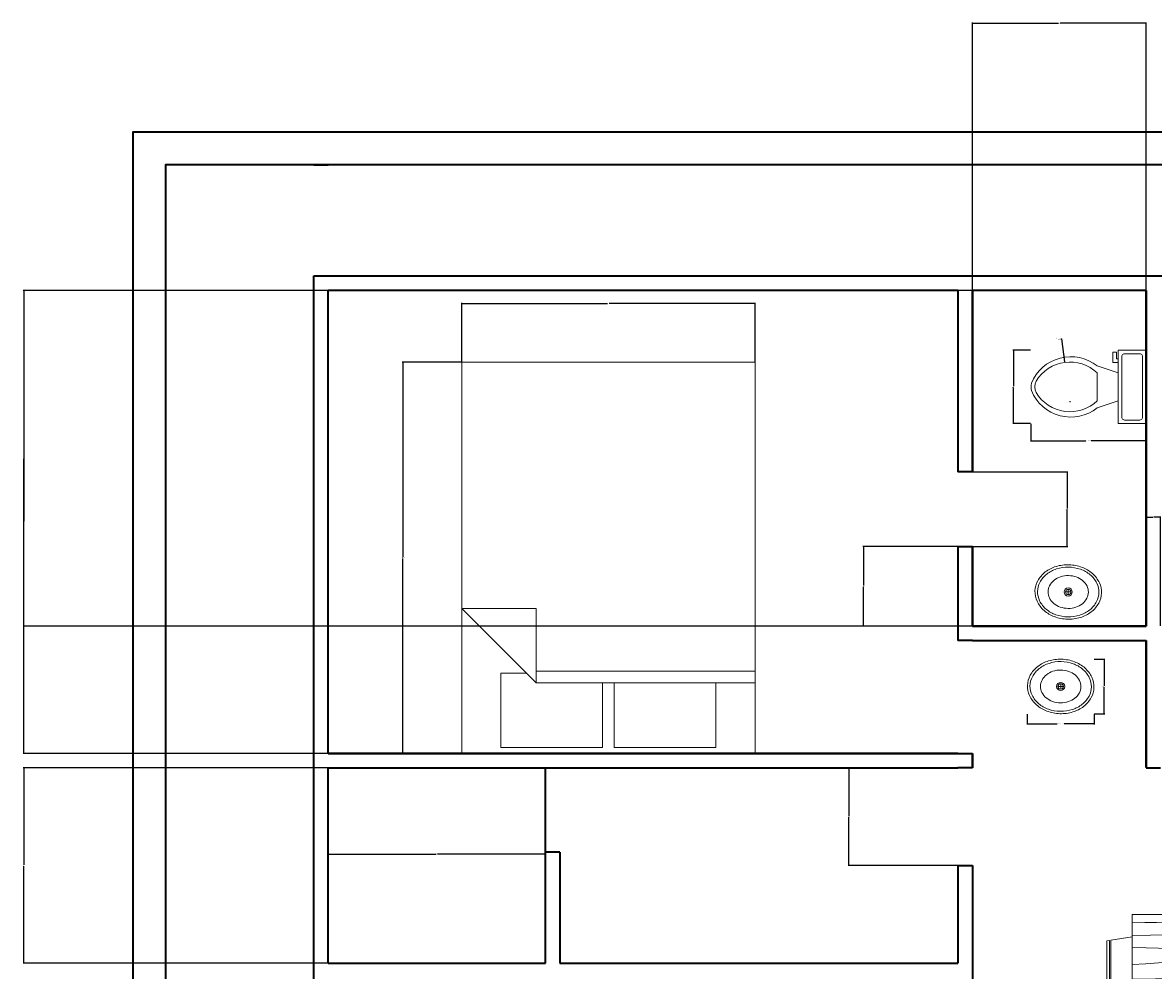
# Model space of a CAD drawing. Units: feet. Extents: x 2335 to 2876, y 491 to 1152.
# Tile 3 of 4: x 2335 to 2648, y 890 to 1152. Entities that reach past the tile are written whole.
import ezdxf

# ---------------------------------------------------------------- set-up
doc = ezdxf.new("R2010")
doc.units = ezdxf.units.FT
for name, color, linetype, lineweight in [('A-ANNO-DIMS', 2, 'Continuous', 18), ('A-FLOR-FIXT', 9, 'Continuous', 18), ('A-FURN', 8, 'Continuous', 18), ('A-WALL', 7, 'Continuous', 35), ('C-PROP', 3, 'Continuous', 35)]:
    doc.layers.add(name, color=color, linetype=linetype, lineweight=lineweight)
doc.styles.get("Standard").update_dxf_attribs({"font": 'arial.ttf'})
doc.dimstyles.get("Standard").update_dxf_attribs({"dimtxt": 0.18, "dimasz": 0.18, "dimexe": 0.18, "dimexo": 0.0625, "dimgap": 0.09, "dimtad": 0, "dimtih": 1, "dimtoh": 1, "dimdec": 4, "dimzin": 0, "dimdsep": 46, "dimlunit": 4, "dimtxsty": 'Standard', "dimcen": 0.09, "dimadec": 0, "dimazin": 0, "dimtfac": 1, "dimtdec": 4, "dimtofl": 0, "dimtmove": 0, "dimatfit": 3, "dimfxl": 1, "dimtolj": 1, "dimtzin": 0, "dimarcsym": 0})

# ---------------------------------------------------------------- blocks, each defined once
blk = doc.blocks.new('Bed - Queen')
for p, q in [((0, -80.00003), (0, 0)), ((0, 0), (59.99999, 0)), ((59.99999, 0), (59.99999, -80.00003)), ((7.99999, -1.2), (28.79998, -1.2)), ((7.99999, -14.4), (7.99999, -1.2)), ((28.79998, -1.2), (28.79998, -14.4)), ((31.19999, -1.2), (51.99999, -1.2)), ((31.19999, -14.4), (31.19999, -1.2)), ((51.99999, -1.2), (51.99999, -16.4)), ((0, -14.4), (44.8, -14.4)), ((59.99999, -29.6), (44.8, -14.4)), ((44.8, -14.4), (44.8, -29.6)), ((44.8, -16.8), (0, -16.8)), ((51.99999, -16.4), (46.79936, -16.4)), ((44.8, -29.6), (59.99999, -29.6)), ((59.99999, -80.00003), (0, -80.00003))]:
    blk.add_line(p, q)
blk = doc.blocks.new('Toilet - top')
for p, q in [((9.5, -6), (9.5, -2)), ((-10, -8.5), (-8, -8.5)), ((-10, -9.5), (-10, -8.5)), ((-7, -9.5), (-10, -9.5)), ((-8, -8.5), (-8, -8)), ((-7, -8), (-7, -9.5)), ((-4, -8), (-6, -14)), ((4, -8), (6, -14)), ((4, -14), (-4, -14))]:
    blk.add_line(p, q)
blk.add_lwpolyline([(10.5, -8), (10.5, 0), (-10.5, 0), (-10.5, -8)], close=True)
for points in [[(-9.5, -2), (-9.5, -6)], [(8.5, -1), (-8.5, -1)], [(-8.5, -7), (8.5, -7)]]:
    blk.add_lwpolyline(points)
for centre, radius, start, end in [((-8.62, -1.88), 0.884, 81.8699, 188.1301), ((8.62, -1.88), 0.884, 351.8699, 98.1301), ((-8.62, -6.12), 0.884, 171.8699, 278.1301), ((8.62, -6.12), 0.884, 261.8699, 8.1301), ((3.52, -21.58), 12.17, 141.4691, 247.9714), ((4.2, -21.82), 11.33, 136.3677, 238.9468), ((-3.52, -21.58), 12.17, 292.0284, 38.5307), ((-4.2, -21.82), 11.33, 301.053, 43.6321), ((0, -27.88), 4, 245.7318, 294.2682), ((0, -29), 4, 254.8605, 285.1395)]:
    blk.add_arc(centre, radius, start, end)
blk = doc.blocks.new('Sink - Oval top')
for p, q in [((-1, 0), (1, 0)), ((0, 1), (0, -1))]:
    blk.add_line(p, q)
for points in [[(-12.23, 0.39, 0.117634), (-11.46, -3.36, 0.104469), (-8.88, -6.8, 0.090016), (-5.08, -9.07, 0.08192), (-0.32, -10.02, 0.08192), (4.49, -9.38, 0.090016), (8.42, -7.36, 0.104469), (11.22, -4.09, 0.117634), (12.23, -0.39, 0.117634), (11.46, 3.36, 0.104469), (8.88, 6.8, 0.090016), (5.08, 9.07, 0.08192), (0.32, 10.02, 0.08192), (-4.49, 9.38, 0.090016), (-8.42, 7.36, 0.104469), (-11.22, 4.09, 0.117634)], [(-11.29, 0.16, 0.118622), (-10.52, -3.25, 0.104678), (-8.07, -6.36, 0.089562), (-4.54, -8.37, 0.081185), (-0.13, -9.15, 0.081185), (4.3, -8.49, 0.089562), (7.89, -6.58, 0.104678), (10.42, -3.55, 0.118622), (11.29, -0.16, 0.118622), (10.52, 3.25, 0.104678), (8.07, 6.36, 0.089562), (4.54, 8.37, 0.081185), (0.13, 9.15, 0.081185), (-4.3, 8.49, 0.089562), (-7.89, 6.58, 0.104678), (-10.42, 3.55, 0.118622)], [(-7.42, 0.08, 0.118283), (-6.91, -2.17, 0.104607), (-5.29, -4.21, 0.089718), (-2.97, -5.53, 0.081436), (-0.07, -6.04, 0.081436), (2.84, -5.59, 0.089718), (5.2, -4.33, 0.104607), (6.86, -2.32, 0.118283), (7.42, -0.08, 0.118283), (6.91, 2.17, 0.104607), (5.29, 4.21, 0.089718), (2.97, 5.53, 0.081436), (0.07, 6.04, 0.081436), (-2.84, 5.59, 0.089718), (-5.2, 4.33, 0.104607), (-6.86, 2.32, 0.118283)]]:
    blk.add_lwpolyline(points, format="xyb", close=True)
for radius in [1.5, 1]:
    blk.add_circle((0, 0), radius)
blk = doc.blocks.new('Dining Set - 36 x 72 in.')
for p, q in [((-22.2343, 26.00059), (-23.4847, 17.99762)), ((-22.2304, 26), (-5.7608, 26)), ((-22, 27.5), (-22.1562, 26.50042)), ((-5.8416, 26.5), (-22.1534, 26.5)), ((-22, 27.5), (-6, 27.5)), ((-5.8437, 26.49966), (-6, 27.5)), ((-4.5152, 17.99762), (-5.7655, 25.99926)), ((5.7657, 26.00059), (4.5153, 17.99762)), ((5.7696, 26), (22.2392, 26)), ((6, 27.5), (5.8438, 26.50042)), ((22.1584, 26.5), (5.8466, 26.5)), ((6, 27.5), (22, 27.5)), ((22.1563, 26.49966), (22, 27.5)), ((23.4848, 17.99762), (22.2345, 25.99926)), ((36, 18), (-36, 18)), ((-36, 18), (-36, -18)), ((36, -18), (36, 18)), ((-44.0006, 8.23428), (-35.9976, 9.48474)), ((44.0006, 8.23428), (35.9976, 9.48474)), ((-45.5, 8), (-44.5004, 8.15617)), ((-45.5, 8), (-45.5, -8)), ((-44.5, -8.15843), (-44.5, 8.15338)), ((-44, 8.23041), (-44, -8.23915)), ((44, 8.23041), (44, -8.23915)), ((44.5, -8.15843), (44.5, 8.15338)), ((45.5, 8), (44.5005, 8.15617)), ((45.5, 8), (45.5, -8)), ((-44.4997, -8.15631), (-45.5, -8)), ((-35.9976, -9.48476), (-43.9993, -8.2345)), ((35.9976, -9.48476), (43.9993, -8.2345)), ((44.4997, -8.15631), (45.5, -8)), ((-36, -18), (36, -18)), ((-22.2343, -26.0006), (-23.4847, -17.99762)), ((-4.5152, -17.99762), (-5.7655, -25.99928)), ((5.7657, -26.0006), (4.5153, -17.99762)), ((23.4848, -17.99762), (22.2345, -25.99928)), ((-22.2304, -26), (-5.7608, -26)), ((-22, -27.5), (-22.1562, -26.50044)), ((-5.8416, -26.5), (-22.1534, -26.5)), ((-22, -27.5), (-6, -27.5)), ((-5.8437, -26.49967), (-6, -27.5)), ((5.7696, -26), (22.2392, -26)), ((6, -27.5), (5.8438, -26.50044)), ((22.1584, -26.5), (5.8466, -26.5)), ((6, -27.5), (22, -27.5)), ((22.1563, -26.49967), (22, -27.5))]:
    blk.add_line(p, q)
for points in [[(-36, 15), (-31.1772, 14.97754), (-26.8079, 14.91406), (-22.8538, 14.81543), (-19.276, 14.6875), (-16.0362, 14.53613), (-13.0957, 14.36718), (-10.4159, 14.18652), (-7.9583, 14), (-5.6904, 13.81315), (-3.6035, 13.63021), (-1.6954, 13.45508), (0.0365, 13.29166), (1.5945, 13.14388), (2.9811, 13.01562), (4.1988, 12.9108), (5.25, 12.83333), (6.1393, 12.78613), (6.8802, 12.76823), (7.4883, 12.77767), (7.9792, 12.8125), (8.3685, 12.87077), (8.6719, 12.95052), (8.9049, 13.0498), (9.0833, 13.16666), (9.2205, 13.29899), (9.3216, 13.44401), (9.3895, 13.59879), (9.4271, 13.76041), (9.4373, 13.92594), (9.4232, 14.09245), (9.3875, 14.257), (9.3333, 14.41666), (9.2638, 14.56917), (9.1836, 14.71484), (9.0975, 14.85465), (9.0104, 14.98958), (8.9272, 15.1206), (8.8529, 15.2487), (8.7922, 15.37483), (8.75, 15.5), (8.7305, 15.62467), (8.7344, 15.74739), (8.7617, 15.86621), (8.8125, 15.97916), (8.8867, 16.08431), (8.9844, 16.17968), (9.1055, 16.26334), (9.25, 16.33333), (9.4189, 16.38802), (9.6172, 16.42708), (9.8506, 16.45052), (10.125, 16.45833), (10.4463, 16.45052), (10.8203, 16.42708), (11.2529, 16.38802), (11.75, 16.33333), (12.3184, 16.26318), (12.9694, 16.17838), (13.7151, 16.07991), (14.5677, 15.96875), (15.5395, 15.84586), (16.6426, 15.71224), (17.8893, 15.56884), (19.2917, 15.41666), (20.859, 15.25667), (22.5879, 15.08984), (24.4721, 14.91715), (26.5052, 14.73958), (28.6809, 14.5581), (30.9929, 14.3737), (33.4347, 14.18733), (36, 14)], [(-36, 10), (-28.9766, 10.14274), (-23.1725, 10.20442), (-18.4241, 10.19775), (-14.5677, 10.13541), (-11.4399, 10.03011), (-8.877, 9.89453), (-6.7154, 9.74137), (-4.7917, 9.58333), (-2.9698, 9.43082), (-1.2246, 9.28515), (0.4415, 9.14534), (2.026, 9.01041), (3.5266, 8.87939), (4.9408, 8.7513), (6.266, 8.62516), (7.5, 8.5), (8.6411, 8.37549), (9.6914, 8.2539), (10.6538, 8.13818), (11.5312, 8.03125), (12.3267, 7.93603), (13.043, 7.85547), (13.6831, 7.79248), (14.25, 7.75), (14.7471, 7.7303), (15.1797, 7.73307), (15.5537, 7.75732), (15.875, 7.80208), (16.1494, 7.86637), (16.3828, 7.94922), (16.5811, 8.04964), (16.75, 8.16666), (16.8944, 8.29915), (17.0143, 8.44531), (17.1089, 8.60319), (17.1771, 8.77083), (17.218, 8.94629), (17.2305, 9.1276), (17.2137, 9.31282), (17.1667, 9.5), (17.0895, 9.6875), (16.987, 9.875), (16.8649, 10.0625), (16.7292, 10.25), (16.5856, 10.4375), (16.4401, 10.625), (16.2985, 10.8125), (16.1667, 11), (16.05, 11.18733), (15.9518, 11.3737), (15.8752, 11.5581), (15.8229, 11.73958), (15.798, 11.91715), (15.8034, 12.08984), (15.842, 12.25667), (15.9167, 12.41666), (16.0295, 12.56836), (16.1784, 12.70833), (16.3605, 12.83268), (16.5729, 12.9375), (16.8127, 13.01888), (17.0768, 13.07291), (17.3625, 13.0957), (17.6667, 13.08333), (17.9894, 13.03312), (18.3418, 12.94726), (18.7382, 12.82918), (19.1927, 12.68229), (19.7195, 12.51001), (20.3327, 12.31575), (21.0465, 12.10294), (21.875, 11.875), (22.8357, 11.63354), (23.959, 11.37304), (25.2786, 11.08618), (26.8282, 10.76562), (28.6414, 10.40405), (30.752, 9.99414), (33.1936, 9.52856), (36, 9)], [(-36, 5.5), (-30.7157, 5.3348), (-26.069, 5.20963), (-21.9946, 5.11767), (-18.4271, 5.05208), (-15.3009, 5.00602), (-12.5508, 4.97265), (-10.1112, 4.94515), (-7.9167, 4.91666), (-5.909, 4.88167), (-4.0586, 4.83984), (-2.3429, 4.79215), (-0.7396, 4.73958), (0.7739, 4.6831), (2.22, 4.6237), (3.6213, 4.56233), (5, 4.5), (6.373, 4.43782), (7.7344, 4.3776), (9.0723, 4.32129), (10.375, 4.27083), (11.6309, 4.22819), (12.8281, 4.19531), (13.9551, 4.17415), (15, 4.16666), (15.954, 4.17448), (16.819, 4.19791), (17.6001, 4.23698), (18.3021, 4.29166), (18.9299, 4.36198), (19.4883, 4.44791), (19.9823, 4.54948), (20.4167, 4.66666), (20.7969, 4.79899), (21.1302, 4.94401), (21.4245, 5.09879), (21.6875, 5.26041), (21.9271, 5.42594), (22.1511, 5.59245), (22.3672, 5.757), (22.5834, 5.91666), (22.8065, 6.06868), (23.0404, 6.21093), (23.2879, 6.34147), (23.5521, 6.45833), (23.8358, 6.55957), (24.142, 6.64323), (24.4735, 6.70735), (24.8334, 6.75), (25.2235, 6.76969), (25.642, 6.76692), (26.0858, 6.74267), (26.5521, 6.69791), (27.0379, 6.63362), (27.5404, 6.55078), (28.0565, 6.45036), (28.5834, 6.33333), (29.1242, 6.19987), (29.7071, 6.04687), (30.3661, 5.87044), (31.1354, 5.66666), (32.0493, 5.43164), (33.142, 5.16146), (34.4475, 4.85221), (36, 4.5)], [(-36, -1), (-30.7915, -0.6591), (-26.0195, -0.38216), (-21.6519, -0.16284), (-17.6563, 0.00521), (-14.0005, 0.12833), (-10.6523, 0.21289), (-7.5796, 0.26522), (-4.75, 0.29166), (-2.134, 0.29793), (0.2878, 0.28711), (2.5317, 0.26163), (4.6146, 0.22396), (6.5529, 0.17651), (8.3633, 0.12174), (10.0623, 0.06209), (11.6667, 0), (13.1899, -0.06201), (14.6341, -0.1211), (15.9982, -0.17432), (17.2813, -0.21875), (18.4823, -0.25147), (19.6003, -0.26953), (20.6343, -0.27002), (21.5834, -0.25), (22.4481, -0.20768), (23.2357, -0.14584), (23.9549, -0.06836), (24.6146, 0.02083), (25.2235, 0.11784), (25.7904, 0.21875), (26.3241, 0.31966), (26.8334, 0.41666), (27.3265, 0.50618), (27.8099, 0.58593), (28.2894, 0.65397), (28.7709, 0.70833), (29.2601, 0.74707), (29.763, 0.76823), (30.2855, 0.76985), (30.8334, 0.75), (31.4088, 0.70784), (31.9994, 0.64713), (32.589, 0.57275), (33.1615, 0.48958), (33.7008, 0.4025), (34.1908, 0.3164), (34.6153, 0.23616), (34.9584, 0.16666), (35.2099, 0.11165), (35.3848, 0.07031), (35.504, 0.04069), (35.5886, 0.02083), (35.6594, 0.00879), (35.7377, 0.0026), (35.8442, 0.00032), (36, 0)], [(-36, -6.5), (-27.1843, -6.31267), (-20.084, -6.1263), (-14.469, -5.9419), (-10.1094, -5.76042), (-6.7752, -5.58285), (-4.2363, -5.41016), (-2.2629, -5.24333), (-0.625, -5.08334), (0.8708, -4.93099), (2.2715, -4.78646), (3.5872, -4.64974), (4.8281, -4.52084), (6.0046, -4.39974), (7.127, -4.28646), (8.2053, -4.18099), (9.25, -4.08334), (10.2705, -3.99382), (11.2734, -3.91407), (12.2647, -3.84603), (13.25, -3.79167), (14.2354, -3.75293), (15.2266, -3.73177), (16.2295, -3.73015), (17.25, -3.75), (18.2912, -3.79248), (19.3451, -3.85547), (20.4009, -3.93604), (21.4479, -4.03125), (22.4754, -4.13819), (23.4727, -4.25391), (24.4289, -4.37549), (25.3334, -4.5), (26.1785, -4.62492), (26.9694, -4.74935), (27.7145, -4.87281), (28.4219, -4.99479), (29.1, -5.11483), (29.7572, -5.23242), (30.4016, -5.34709), (31.0417, -5.45834), (31.6837, -5.56437), (32.3262, -5.65821), (32.9658, -5.73153), (33.599, -5.77604), (34.2224, -5.78345), (34.8327, -5.74545), (35.4264, -5.65373), (36, -5.5)], [(-36, -10), (-26.4022, -9.81299), (-18.4675, -9.62891), (-11.9839, -9.45069), (-6.7396, -9.28125), (-2.5226, -9.12354), (0.8789, -8.98047), (3.6769, -8.85498), (6.0833, -8.75), (8.2767, -8.66765), (10.3021, -8.60677), (12.1712, -8.56543), (13.8958, -8.54167), (15.4876, -8.53353), (16.9583, -8.53907), (18.3197, -8.55632), (19.5834, -8.58334), (20.7616, -8.61841), (21.8685, -8.66081), (22.9188, -8.71004), (23.9271, -8.76563), (24.9081, -8.82707), (25.8763, -8.89388), (26.8465, -8.96558), (27.8334, -9.04167), (28.8474, -9.12118), (29.8828, -9.20117), (30.93, -9.27824), (31.9792, -9.34896), (33.0205, -9.40991), (34.0443, -9.45768), (35.0407, -9.48885), (36, -9.5)], [(-36, -14.5), (-30.0881, -14.33513), (-25.0332, -14.21224), (-20.7312, -14.12647), (-17.0781, -14.07292), (-13.97, -14.04671), (-11.3027, -14.04297), (-8.9724, -14.05681), (-6.875, -14.08334), (-4.9224, -14.11833), (-3.0905, -14.16016), (-1.3709, -14.20785), (0.2448, -14.26042), (1.7647, -14.3169), (3.1973, -14.3763), (4.5507, -14.43767), (5.8333, -14.5), (7.0554, -14.5621), (8.235, -14.62175), (9.3922, -14.67652), (10.5469, -14.72396), (11.7192, -14.76164), (12.929, -14.78711), (14.1965, -14.79794), (15.5417, -14.79167), (16.9933, -14.76424), (18.6152, -14.70508), (20.4804, -14.60197), (22.6615, -14.44271), (25.2312, -14.21509), (28.2624, -13.9069), (31.8277, -13.50594), (36, -13)]]:
    blk.add_lwpolyline(points)
blk = doc.blocks.new('*D8')
at = {"layer": 'A-ANNO-DIMS', "color": 0, "lineweight": -2, "transparency": 16777216}
for p, q in [((2456.6, 1057.92), (2440.26, 1057.92)), ((2440.44, 1057.74), (2440.44, 1004.04)), ((2440.44, 949.98), (2440.44, 1003.68)), ((2456.6, 949.8), (2440.26, 949.8))]:
    blk.add_line(p, q, dxfattribs=at)
at = {"layer": 'A-ANNO-DIMS', "color": 0, "transparency": 16777216}
for points in [[(2440.41, 1057.74), (2440.47, 1057.74), (2440.44, 1057.92)], [(2440.41, 949.98), (2440.47, 949.98), (2440.44, 949.8)]]:
    blk.add_solid(points, dxfattribs=at)
at = {"layer": 'Defpoints', "color": 0, "transparency": 16777216}
for p in [(2456.66, 1057.92), (2440.44, 949.8), (2456.66, 949.8)]:
    blk.add_point(p, dxfattribs=at)
at = {"layer": 'A-ANNO-DIMS', "color": 0, "transparency": 16777216, "insert": (2440.44, 1003.86), "char_height": 0.18, "attachment_point": 5}
blk.add_mtext('\\A1;BED 108', dxfattribs=at)
blk = doc.blocks.new('*D9')
at = {"layer": 'A-ANNO-DIMS', "color": 0, "lineweight": -2, "transparency": 16777216}
for p, q in [((2456.66, 1057.98), (2456.66, 1074.31)), ((2456.84, 1074.13), (2497, 1074.13)), ((2537.57, 1074.13), (2497.41, 1074.13)), ((2537.75, 1057.98), (2537.75, 1074.31))]:
    blk.add_line(p, q, dxfattribs=at)
at = {"layer": 'A-ANNO-DIMS', "color": 0, "transparency": 16777216}
for points in [[(2456.84, 1074.16), (2456.84, 1074.1), (2456.66, 1074.13)], [(2537.57, 1074.16), (2537.57, 1074.1), (2537.75, 1074.13)]]:
    blk.add_solid(points, dxfattribs=at)
at = {"layer": 'Defpoints', "color": 0, "transparency": 16777216}
for p in [(2456.66, 1074.13), (2456.66, 1057.92), (2537.75, 1057.92)]:
    blk.add_point(p, dxfattribs=at)
at = {"layer": 'A-ANNO-DIMS', "color": 0, "transparency": 16777216, "insert": (2497.21, 1074.13), "char_height": 0.18, "attachment_point": 5}
blk.add_mtext('\\A1;81', dxfattribs=at)
blk = doc.blocks.new('*D12')
at = {"layer": 'A-ANNO-DIMS', "color": 0, "lineweight": -2, "transparency": 16777216}
for p, q in [((2612.96, 960.67), (2612.96, 957.78)), ((2631.41, 960.67), (2631.41, 957.78)), ((2613.14, 957.96), (2621.25, 957.96)), ((2631.23, 957.96), (2623.12, 957.96))]:
    blk.add_line(p, q, dxfattribs=at)
at = {"layer": 'A-ANNO-DIMS', "color": 0, "transparency": 16777216}
for points in [[(2613.14, 957.99), (2613.14, 957.93), (2612.96, 957.96)], [(2631.23, 957.99), (2631.23, 957.93), (2631.41, 957.96)]]:
    blk.add_solid(points, dxfattribs=at)
at = {"layer": 'Defpoints', "color": 0, "transparency": 16777216}
for p in [(2612.96, 960.73), (2631.41, 960.73), (2631.41, 957.96)]:
    blk.add_point(p, dxfattribs=at)
at = {"layer": 'A-ANNO-DIMS', "color": 0, "transparency": 16777216, "insert": (2622.19, 957.96), "char_height": 0.18, "attachment_point": 5}
blk.add_mtext('\\A1;BASIN 18 TYP.', dxfattribs=at)
blk = doc.blocks.new('*D13')
at = {"layer": 'A-ANNO-DIMS', "color": 0, "lineweight": -2, "transparency": 16777216}
for p, q in [((2631.47, 975.86), (2634.36, 975.86)), ((2634.18, 975.68), (2634.18, 968.48)), ((2634.18, 960.91), (2634.18, 968.12)), ((2631.47, 960.73), (2634.36, 960.73))]:
    blk.add_line(p, q, dxfattribs=at)
at = {"layer": 'A-ANNO-DIMS', "color": 0, "transparency": 16777216}
for points in [[(2634.15, 975.68), (2634.21, 975.68), (2634.18, 975.86)], [(2634.15, 960.91), (2634.21, 960.91), (2634.18, 960.73)]]:
    blk.add_solid(points, dxfattribs=at)
at = {"layer": 'Defpoints', "color": 0, "transparency": 16777216}
for p in [(2631.41, 975.86), (2634.18, 975.86), (2631.41, 960.73)]:
    blk.add_point(p, dxfattribs=at)
at = {"layer": 'A-ANNO-DIMS', "color": 0, "transparency": 16777216, "insert": (2634.18, 968.3), "char_height": 0.18, "attachment_point": 5}
blk.add_mtext('\\A1;15 TYP.', dxfattribs=at)
blk = doc.blocks.new('*D14')
at = {"layer": 'A-ANNO-DIMS', "color": 0, "lineweight": -2, "transparency": 16777216}
for p, q in [((2613.94, 1040.92), (2613.94, 1036.03)), ((2645.8, 1040.92), (2645.8, 1036.03)), ((2614.12, 1036.21), (2629.09, 1036.21)), ((2645.62, 1036.21), (2630.64, 1036.21))]:
    blk.add_line(p, q, dxfattribs=at)
at = {"layer": 'A-ANNO-DIMS', "color": 0, "transparency": 16777216}
for points in [[(2614.12, 1036.24), (2614.12, 1036.18), (2613.94, 1036.21)], [(2645.62, 1036.24), (2645.62, 1036.18), (2645.8, 1036.21)]]:
    blk.add_solid(points, dxfattribs=at)
at = {"layer": 'Defpoints', "color": 0, "transparency": 16777216}
for p in [(2613.94, 1040.98), (2645.8, 1040.98), (2645.8, 1036.21)]:
    blk.add_point(p, dxfattribs=at)
at = {"layer": 'A-ANNO-DIMS', "color": 0, "transparency": 16777216, "insert": (2629.87, 1036.21), "char_height": 0.18, "attachment_point": 5}
blk.add_mtext('\\A1;WC 32 TYP.', dxfattribs=at)
blk = doc.blocks.new('*D15')
at = {"layer": 'A-ANNO-DIMS', "color": 0, "lineweight": -2, "transparency": 16777216}
for p, q in [((2613.87, 1061.23), (2608.98, 1061.23)), ((2609.16, 1061.05), (2609.16, 1051.29)), ((2609.16, 1041.16), (2609.16, 1050.93)), ((2613.87, 1040.98), (2608.98, 1040.98))]:
    blk.add_line(p, q, dxfattribs=at)
at = {"layer": 'A-ANNO-DIMS', "color": 0, "transparency": 16777216}
for points in [[(2609.13, 1061.05), (2609.19, 1061.05), (2609.16, 1061.23)], [(2609.13, 1041.16), (2609.19, 1041.16), (2609.16, 1040.98)]]:
    blk.add_solid(points, dxfattribs=at)
at = {"layer": 'Defpoints', "color": 0, "transparency": 16777216}
for p in [(2613.94, 1061.23), (2609.16, 1040.98), (2613.94, 1040.98)]:
    blk.add_point(p, dxfattribs=at)
at = {"layer": 'A-ANNO-DIMS', "color": 0, "transparency": 16777216, "insert": (2609.16, 1051.11), "char_height": 0.18, "attachment_point": 5}
blk.add_mtext('\\A1;20 TYP.', dxfattribs=at)
blk = doc.blocks.new('*D50')
at = {"layer": 'A-ANNO-DIMS', "color": 0, "lineweight": -2, "transparency": 16777216}
for p, q in [((2419.73, 945.8), (2335.47, 945.8)), ((2335.65, 945.62), (2335.65, 918.98)), ((2335.65, 891.98), (2335.65, 918.62)), ((2419.73, 891.8), (2335.47, 891.8))]:
    blk.add_line(p, q, dxfattribs=at)
at = {"layer": 'A-ANNO-DIMS', "color": 0, "transparency": 16777216}
for points in [[(2335.62, 945.62), (2335.68, 945.62), (2335.65, 945.8)], [(2335.62, 891.98), (2335.68, 891.98), (2335.65, 891.8)]]:
    blk.add_solid(points, dxfattribs=at)
at = {"layer": 'Defpoints', "color": 0, "transparency": 16777216}
for p in [(2335.65, 945.8), (2419.8, 945.8), (2419.8, 891.8)]:
    blk.add_point(p, dxfattribs=at)
at = {"layer": 'A-ANNO-DIMS', "color": 0, "transparency": 16777216, "insert": (2335.65, 918.8), "char_height": 0.18, "attachment_point": 5}
blk.add_mtext('\\A1;54', dxfattribs=at)
blk = doc.blocks.new('*D51')
at = {"layer": 'A-ANNO-DIMS', "color": 0, "lineweight": -2, "transparency": 16777216}
for p, q in [((2419.8, 891.86), (2419.8, 922.13)), ((2419.98, 921.95), (2449.58, 921.95)), ((2479.62, 921.95), (2450.02, 921.95)), ((2479.8, 891.86), (2479.8, 922.13))]:
    blk.add_line(p, q, dxfattribs=at)
at = {"layer": 'A-ANNO-DIMS', "color": 0, "transparency": 16777216}
for points in [[(2419.98, 921.98), (2419.98, 921.92), (2419.8, 921.95)], [(2479.62, 921.98), (2479.62, 921.92), (2479.8, 921.95)]]:
    blk.add_solid(points, dxfattribs=at)
at = {"layer": 'Defpoints', "color": 0, "transparency": 16777216}
for p in [(2479.8, 921.95), (2419.8, 891.8), (2479.8, 891.8)]:
    blk.add_point(p, dxfattribs=at)
at = {"layer": 'A-ANNO-DIMS', "color": 0, "transparency": 16777216, "insert": (2449.8, 921.95), "char_height": 0.18, "attachment_point": 5}
blk.add_mtext('\\A1;60', dxfattribs=at)
blk = doc.blocks.new('*D52')
at = {"layer": 'A-ANNO-DIMS', "color": 0, "lineweight": -2, "transparency": 16777216}
for p, q in [((2593.73, 945.8), (2563.47, 945.8)), ((2563.65, 945.62), (2563.65, 932.48)), ((2563.65, 918.98), (2563.65, 932.12)), ((2593.73, 918.8), (2563.47, 918.8))]:
    blk.add_line(p, q, dxfattribs=at)
at = {"layer": 'A-ANNO-DIMS', "color": 0, "transparency": 16777216}
for points in [[(2563.62, 945.62), (2563.68, 945.62), (2563.65, 945.8)], [(2563.62, 918.98), (2563.68, 918.98), (2563.65, 918.8)]]:
    blk.add_solid(points, dxfattribs=at)
at = {"layer": 'Defpoints', "color": 0, "transparency": 16777216}
for p in [(2563.65, 945.8), (2593.8, 945.8), (2593.8, 918.8)]:
    blk.add_point(p, dxfattribs=at)
at = {"layer": 'A-ANNO-DIMS', "color": 0, "transparency": 16777216, "insert": (2563.65, 932.3), "char_height": 0.18, "attachment_point": 5}
blk.add_mtext('\\A1;27', dxfattribs=at)
blk = doc.blocks.new('*D53')
at = {"layer": 'A-ANNO-DIMS', "color": 0, "lineweight": -2, "transparency": 16777216}
for p, q in [((2419.74, 1077.8), (2335.47, 1077.8)), ((2335.65, 1077.62), (2335.65, 1013.98)), ((2335.65, 949.98), (2335.65, 1013.62)), ((2419.73, 949.8), (2335.47, 949.8))]:
    blk.add_line(p, q, dxfattribs=at)
at = {"layer": 'A-ANNO-DIMS', "color": 0, "transparency": 16777216}
for points in [[(2335.62, 1077.62), (2335.68, 1077.62), (2335.65, 1077.8)], [(2335.62, 949.98), (2335.68, 949.98), (2335.65, 949.8)]]:
    blk.add_solid(points, dxfattribs=at)
at = {"layer": 'Defpoints', "color": 0, "transparency": 16777216}
for p in [(2335.65, 1077.8), (2419.8, 1077.8), (2419.8, 949.8)]:
    blk.add_point(p, dxfattribs=at)
at = {"layer": 'A-ANNO-DIMS', "color": 0, "transparency": 16777216, "insert": (2335.65, 1013.8), "char_height": 0.18, "attachment_point": 5}
blk.add_mtext('\\A1;128', dxfattribs=at)
blk = doc.blocks.new('*D55')
at = {"layer": 'A-ANNO-DIMS', "color": 0, "lineweight": -2, "transparency": 16777216}
for p, q in [((2597.8, 1077.86), (2597.8, 1151.82)), ((2597.98, 1151.64), (2621.57, 1151.64)), ((2645.62, 1151.64), (2622.02, 1151.64)), ((2645.8, 1077.86), (2645.8, 1151.82))]:
    blk.add_line(p, q, dxfattribs=at)
at = {"layer": 'A-ANNO-DIMS', "color": 0, "transparency": 16777216}
for points in [[(2597.98, 1151.67), (2597.98, 1151.61), (2597.8, 1151.64)], [(2645.62, 1151.67), (2645.62, 1151.61), (2645.8, 1151.64)]]:
    blk.add_solid(points, dxfattribs=at)
at = {"layer": 'Defpoints', "color": 0, "transparency": 16777216}
for p in [(2645.8, 1151.64), (2597.8, 1077.8), (2645.8, 1077.8)]:
    blk.add_point(p, dxfattribs=at)
at = {"layer": 'A-ANNO-DIMS', "color": 0, "transparency": 16777216, "insert": (2621.8, 1151.64), "char_height": 0.18, "attachment_point": 5}
blk.add_mtext('\\A1;48', dxfattribs=at)
blk = doc.blocks.new('*D57')
at = {"layer": 'A-ANNO-DIMS', "color": 0, "lineweight": -2, "transparency": 16777216}
for p, q in [((2645.8, 985.02), (2645.8, 1015.28)), ((2645.98, 1015.1), (2647.65, 1015.1)), ((2649.62, 1015.1), (2647.95, 1015.1)), ((2649.8, 985.02), (2649.8, 1015.28))]:
    blk.add_line(p, q, dxfattribs=at)
at = {"layer": 'A-ANNO-DIMS', "color": 0, "transparency": 16777216}
for points in [[(2645.98, 1015.13), (2645.98, 1015.07), (2645.8, 1015.1)], [(2649.62, 1015.13), (2649.62, 1015.07), (2649.8, 1015.1)]]:
    blk.add_solid(points, dxfattribs=at)
at = {"layer": 'Defpoints', "color": 0, "transparency": 16777216}
for p in [(2649.8, 1015.1), (2645.8, 984.95), (2649.8, 984.95)]:
    blk.add_point(p, dxfattribs=at)
at = {"layer": 'A-ANNO-DIMS', "color": 0, "transparency": 16777216, "insert": (2647.8, 1015.1), "char_height": 0.18, "attachment_point": 5}
blk.add_mtext('\\A1;4', dxfattribs=at)
blk = doc.blocks.new('*D58')
at = {"layer": 'A-ANNO-DIMS', "color": 0, "lineweight": -2, "transparency": 16777216}
for p, q in [((2597.73, 1077.8), (2335.47, 1077.8)), ((2335.65, 1077.62), (2335.65, 1031.56)), ((2335.65, 985.13), (2335.65, 1031.19)), ((2597.73, 984.95), (2335.47, 984.95))]:
    blk.add_line(p, q, dxfattribs=at)
at = {"layer": 'A-ANNO-DIMS', "color": 0, "transparency": 16777216}
for points in [[(2335.62, 1077.62), (2335.68, 1077.62), (2335.65, 1077.8)], [(2335.62, 985.13), (2335.68, 985.13), (2335.65, 984.95)]]:
    blk.add_solid(points, dxfattribs=at)
at = {"layer": 'Defpoints', "color": 0, "transparency": 16777216}
for p in [(2335.65, 1077.8), (2597.8, 1077.8), (2597.8, 984.95)]:
    blk.add_point(p, dxfattribs=at)
at = {"layer": 'A-ANNO-DIMS', "color": 0, "transparency": 16777216, "insert": (2335.65, 1031.38), "char_height": 0.18, "attachment_point": 5}
blk.add_mtext('\\A1;92.84', dxfattribs=at)
blk = doc.blocks.new('*D64')
at = {"layer": 'A-ANNO-DIMS', "color": 0, "lineweight": -2, "transparency": 16777216}
for p, q in [((2593.86, 1027.59), (2624.13, 1027.59)), ((2623.95, 1027.41), (2623.95, 1017.47)), ((2623.95, 1007.17), (2623.95, 1017.11)), ((2593.86, 1006.99), (2624.13, 1006.99))]:
    blk.add_line(p, q, dxfattribs=at)
at = {"layer": 'A-ANNO-DIMS', "color": 0, "transparency": 16777216}
for points in [[(2623.92, 1027.41), (2623.98, 1027.41), (2623.95, 1027.59)], [(2623.92, 1007.17), (2623.98, 1007.17), (2623.95, 1006.99)]]:
    blk.add_solid(points, dxfattribs=at)
at = {"layer": 'Defpoints', "color": 0, "transparency": 16777216}
for p in [(2593.8, 1027.59), (2593.8, 1006.99), (2623.95, 1006.99)]:
    blk.add_point(p, dxfattribs=at)
at = {"layer": 'A-ANNO-DIMS', "color": 0, "transparency": 16777216, "insert": (2623.95, 1017.29), "char_height": 0.18, "attachment_point": 5}
blk.add_mtext('\\A1;20.597', dxfattribs=at)
blk = doc.blocks.new('*D67')
at = {"layer": 'A-ANNO-DIMS', "color": 0, "lineweight": -2, "transparency": 16777216}
for p, q in [((2597.73, 1006.99), (2567.47, 1006.99)), ((2567.65, 1006.81), (2567.65, 996.16)), ((2567.65, 985.13), (2567.65, 995.79)), ((2597.73, 984.95), (2567.47, 984.95))]:
    blk.add_line(p, q, dxfattribs=at)
at = {"layer": 'A-ANNO-DIMS', "color": 0, "transparency": 16777216}
for points in [[(2567.62, 1006.81), (2567.68, 1006.81), (2567.65, 1006.99)], [(2567.62, 985.13), (2567.68, 985.13), (2567.65, 984.95)]]:
    blk.add_solid(points, dxfattribs=at)
at = {"layer": 'Defpoints', "color": 0, "transparency": 16777216}
for p in [(2567.65, 1006.99), (2597.8, 1006.99), (2597.8, 984.95)]:
    blk.add_point(p, dxfattribs=at)
at = {"layer": 'A-ANNO-DIMS', "color": 0, "transparency": 16777216, "insert": (2567.65, 995.97), "char_height": 0.18, "attachment_point": 5}
blk.add_mtext('\\A1;22.04', dxfattribs=at)
blk = doc.blocks.new('*D69')
at = {"layer": 'A-ANNO-DIMS', "color": 0, "lineweight": -2, "transparency": 16777216}
for p, q in [((2622.25, 1064.38), (2622.43, 1064.38)), ((2622.43, 1064.38), (2623.28, 1058.06)), ((2624.67, 1047.06), (2624.85, 1047.06)), ((2624.76, 1046.97), (2624.76, 1047.15))]:
    blk.add_line(p, q, dxfattribs=at)
at = {"layer": 'A-ANNO-DIMS', "color": 0, "transparency": 16777216}
blk.add_solid([(2623.31, 1058.07), (2623.25, 1058.06), (2623.31, 1057.88)], dxfattribs=at)
at = {"layer": 'Defpoints', "color": 0, "transparency": 16777216}
for p in [(2623.31, 1057.88), (2624.76, 1047.06)]:
    blk.add_point(p, dxfattribs=at)
at = {"layer": 'A-ANNO-DIMS', "color": 0, "transparency": 16777216, "insert": (2621.51, 1064.38), "char_height": 0.18, "attachment_point": 5}
blk.add_mtext('\\A1;4X R10.923', dxfattribs=at)

msp = doc.modelspace()

# ---------------------------------------------------------------- linework, layer by layer
at = {"layer": 'A-WALL'}
for p, q in [((2415.7974, 855.7568), (2415.7974, 1081.7975)), ((2415.7974, 1081.7975), (2697.7974, 1081.7975)), ((2593.7974, 1077.7977), (2419.7973, 1077.798)), ((2419.7974, 949.7975), (2419.7976, 1077.798)), ((2593.7974, 1077.7977), (2593.7974, 1027.5899)), ((2593.7974, 1077.7977), (2593.7974, 1027.5899)), ((2593.7974, 1077.7977), (2593.7974, 1027.5899)), ((2597.7974, 1077.7977), (2597.7974, 1027.5899)), ((2645.7974, 1077.7976), (2597.7974, 1077.7977)), ((2597.7974, 1027.5899), (2597.7974, 1077.7977)), ((2645.7974, 984.9529), (2645.7974, 1077.7976)), ((2645.7974, 1077.7976), (2645.7974, 984.9529)), ((2645.7974, 1077.7976), (2645.7974, 984.9529)), ((2645.7974, 1077.7976), (2645.7974, 984.9529)), ((2597.7974, 1027.5899), (2593.7974, 1027.5899)), ((2593.7974, 1006.9934), (2597.7974, 1006.9934)), ((2593.7974, 1006.9934), (2593.7974, 980.9529)), ((2593.7974, 1006.9934), (2593.7974, 980.9529)), ((2593.7974, 1006.9934), (2593.7974, 980.9529)), ((2597.7974, 984.9529), (2597.7974, 1006.9934)), ((2597.7974, 1006.9934), (2597.7974, 984.9529)), ((2645.7974, 984.9529), (2597.7974, 984.9529)), ((2597.7974, 984.9529), (2645.7974, 984.9529)), ((2645.7974, 984.9529), (2597.7974, 984.9529)), ((2597.7974, 984.9529), (2645.7974, 984.9529)), ((2597.7974, 980.9529), (2593.7974, 980.9529)), ((2597.7974, 980.9529), (2645.7974, 980.9529)), ((2597.7974, 980.9529), (2645.7974, 980.9529)), ((2597.7974, 980.9529), (2645.7974, 980.9529)), ((2645.7974, 945.9689), (2645.7974, 980.9529)), ((2645.7974, 980.9529), (2645.7974, 949.7975)), ((2645.7974, 980.9529), (2645.7974, 945.7975)), ((2645.7974, 980.9529), (2645.7974, 949.7975)), ((2593.7974, 949.7975), (2419.7974, 949.7975)), ((2419.7974, 949.7975), (2593.7974, 949.7975)), ((2593.7974, 949.7975), (2419.7974, 949.7975)), ((2593.7974, 949.7975), (2597.7974, 949.7975)), ((2597.7974, 945.7975), (2597.7974, 949.7975)), ((2597.7974, 949.7975), (2597.7974, 945.7975)), ((2597.7974, 949.7975), (2597.7974, 945.7975)), ((2419.7969, 891.7975), (2419.7969, 945.7975)), ((2419.7974, 945.7975), (2593.7974, 945.7975)), ((2419.7974, 945.7975), (2593.7974, 945.7975)), ((2479.7974, 891.7975), (2479.7974, 945.7975)), ((2597.7974, 945.7975), (2593.7974, 945.7975)), ((2645.7974, 945.7975), (2649.7974, 945.7975)), ((2483.7974, 922.4546), (2479.7974, 922.4546)), ((2483.7974, 922.4546), (2483.7974, 891.7975)), ((2593.7974, 918.7975), (2593.7974, 891.7975)), ((2593.7974, 918.7975), (2597.7974, 918.7975)), ((2597.7974, 918.7975), (2597.7974, 614.2261)), ((2419.7974, 891.7975), (2479.7974, 891.7975)), ((2483.7974, 891.7975), (2593.7974, 891.7975))]:
    msp.add_line(p, q, dxfattribs=at)
at = {"layer": 'C-PROP'}
for p, q in [((2374.7967, 1112.4872), (2374.7967, 1081.7975)), ((2415.7974, 1112.4872), (2419.7974, 1112.4872))]:
    msp.add_line(p, q, dxfattribs=at)
msp.add_lwpolyline([(2845.7967, 521.4872), (2845.7967, 1121.4872), (2365.7967, 1121.4872), (2365.7967, 521.4872)], close=True, dxfattribs=at)
msp.add_lwpolyline([(2697.7974, 1112.4872), (2374.7967, 1112.4872), (2374.7967, 530.4872), (2593.7974, 530.4872)], dxfattribs=at)

# ---------------------------------------------------------------- block references
at = {"layer": 'A-FLOR-FIXT', "xscale": 0.9641315578102057, "yscale": 0.9641315578102057, "zscale": 0.9641315578102057, "rotation": 270}
msp.add_blockref('Toilet - top', (2645.7974, 1051.1075), dxfattribs=at)
at = {"layer": 'A-FLOR-FIXT', "xscale": 0.7514563269629554, "yscale": 0.7514563269629554, "zscale": 0.7514563269629554}
for p in [(2624.2621, 994.4081), (2622.1863, 968.2974)]:
    msp.add_blockref('Sink - Oval top', p, dxfattribs=at)
at = {"layer": 'A-FURN', "xscale": 1.35149041109511, "yscale": 1.35149041109511, "zscale": 1.35149041109511, "rotation": 180}
msp.add_blockref('Bed - Queen', (2537.7499, 949.7975), dxfattribs=at)
at = {"layer": 'A-FURN', "xscale": 0.7311477324397611, "yscale": 0.7311477324397611, "zscale": 0.7311477324397611}
msp.add_blockref('Dining Set - 36 x 72 in.', (2668.2264, 892.1257), dxfattribs=at)

# ---------------------------------------------------------------- dimensions: what is measured, and where the dimension line sits
at = {"layer": 'A-ANNO-DIMS'}
for base, p1, p2, picture, middle in [((2645.7974, 1151.6372), (2597.7974, 1077.7977), (2645.7974, 1077.7976), '*D55', (2621.7974, 1151.6372)), ((2649.7974, 1015.1029), (2645.7974, 984.9529), (2649.7974, 984.9529), '*D57', (2647.7974, 1015.1029)), ((2479.7974, 921.9475), (2419.7974, 891.7975), (2479.7974, 891.7975), '*D51', (2449.7974, 921.9475))]:
    dim = msp.add_linear_dim(base=base, p1=p1, p2=p2, dimstyle='Standard', override={"dimdec": 0, "dimlfac": 1, "dimrnd": 0, "dimzin": 0, "dimdsep": 46, "dimlunit": 2}, dxfattribs=at)
    dim.commit()
    dim.dimension.update_dxf_attribs({"geometry": picture, "text_midpoint": middle})
for base, p1, p2, angle, override, picture, middle in [((2335.6467, 1077.7977), (2597.7974, 984.9529), (2597.7974, 1077.7977), 90, {"dimdec": 2, "dimlfac": 1, "dimrnd": 0, "dimzin": 0, "dimdsep": 46, "dimlunit": 2}, '*D58', (2335.6467, 1031.3753)), ((2335.6467, 1077.798), (2419.7974, 949.7975), (2419.7976, 1077.798), 90, {"dimdec": 0, "dimlfac": 1, "dimrnd": 0, "dimzin": 0, "dimdsep": 46, "dimlunit": 2}, '*D53', (2335.6467, 1013.7978)), ((2456.6605, 1074.1347), (2537.7499, 1057.9168), (2456.6605, 1057.9168), 180, {"dimdec": 0, "dimlfac": 1, "dimrnd": 0, "dimzin": 0, "dimdsep": 46, "dimlunit": 2}, '*D9', (2497.2052, 1074.1347)), ((2623.94739, 1006.99339), (2593.79739, 1027.58992), (2593.79739, 1006.99339), 270, {"dimdec": 3, "dimlfac": 1, "dimrnd": 0, "dimzin": 0, "dimdsep": 46, "dimlunit": 2}, '*D64', (2623.94739, 1017.29165)), ((2567.6474, 1006.9934), (2597.7974, 984.9529), (2597.7974, 1006.9934), 90, {"dimdec": 2, "dimlfac": 1, "dimrnd": 0, "dimzin": 0, "dimdsep": 46, "dimlunit": 2}, '*D67', (2567.6474, 995.9731)), ((2335.6467, 945.7975), (2419.7974, 891.7975), (2419.7974, 945.7975), 90, {"dimdec": 0, "dimlfac": 1, "dimrnd": 0, "dimzin": 0, "dimdsep": 46, "dimlunit": 2}, '*D50', (2335.6467, 918.7975)), ((2563.6474, 945.7975), (2593.7974, 918.7975), (2593.7974, 945.7975), 90, {"dimdec": 0, "dimlfac": 1, "dimrnd": 0, "dimzin": 0, "dimdsep": 46, "dimlunit": 2}, '*D52', (2563.6474, 932.2975))]:
    dim = msp.add_linear_dim(base=base, p1=p1, p2=p2, angle=angle, dimstyle='Standard', override=override, dxfattribs=at)
    dim.commit()
    dim.dimension.update_dxf_attribs({"geometry": picture, "text_midpoint": middle})
dim = msp.add_radius_dim(center=(2624.7625, 1047.0582), mpoint=(2623.307, 1057.8836), text='4X <>', dimstyle='Standard', override={"dimdec": 3, "dimlfac": 1, "dimrnd": 0, "dimzin": 0, "dimdsep": 46, "dimlunit": 2}, dxfattribs=at)
dim.commit()
dim.dimension.update_dxf_attribs({"geometry": '*D69', "text_midpoint": (2621.507, 1064.3789), "dimtype": 164})
for base, p1, p2, angle, text, picture, middle in [((2609.1573, 1040.9842), (2613.9365, 1061.2309), (2613.9365, 1040.9842), 270, '<> TYP.', '*D15', (2609.1573, 1051.1075)), ((2440.4426, 949.7975), (2456.6605, 1057.9168), (2456.6605, 949.7975), 270, 'BED <>', '*D8', (2440.4426, 1003.8571)), ((2634.1781, 975.8633), (2631.4107, 960.7315), (2631.4107, 975.8633), 90, '<> TYP.', '*D13', (2634.1781, 968.2974))]:
    dim = msp.add_linear_dim(base=base, p1=p1, p2=p2, angle=angle, text=text, dimstyle='Standard', override={"dimdec": 0, "dimlfac": 1, "dimrnd": 0, "dimzin": 0, "dimdsep": 46, "dimlunit": 2}, dxfattribs=at)
    dim.commit()
    dim.dimension.update_dxf_attribs({"geometry": picture, "text_midpoint": middle})
for base, p1, p2, text, picture, middle in [((2645.7974, 1036.205), (2613.9365, 1040.9842), (2645.7974, 1040.9842), 'WC <> TYP.', '*D14', (2629.8669, 1036.205)), ((2631.4107, 957.9642), (2612.9618, 960.7315), (2631.4107, 960.7315), 'BASIN <> TYP.', '*D12', (2622.1863, 957.9642))]:
    dim = msp.add_linear_dim(base=base, p1=p1, p2=p2, text=text, dimstyle='Standard', override={"dimdec": 0, "dimlfac": 1, "dimrnd": 0, "dimzin": 0, "dimdsep": 46, "dimlunit": 2}, dxfattribs=at)
    dim.commit()
    dim.dimension.update_dxf_attribs({"geometry": picture, "text_midpoint": middle})

doc.saveas('drawing.dxf')
